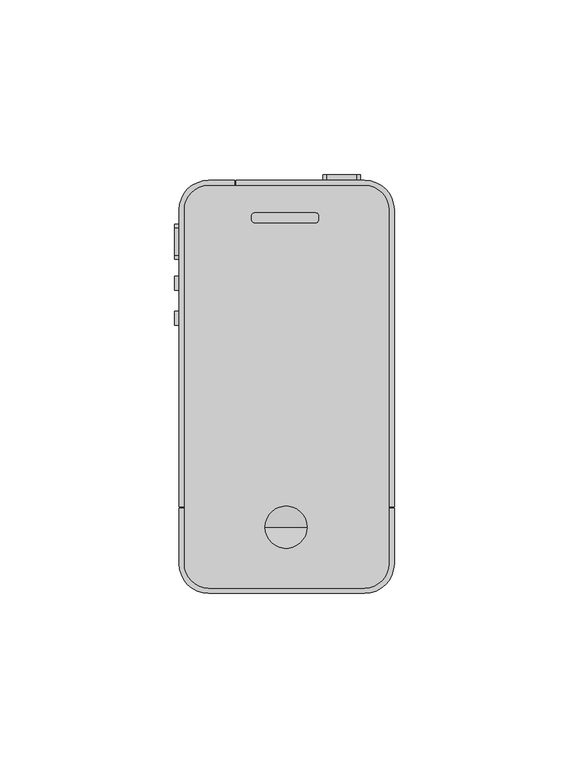
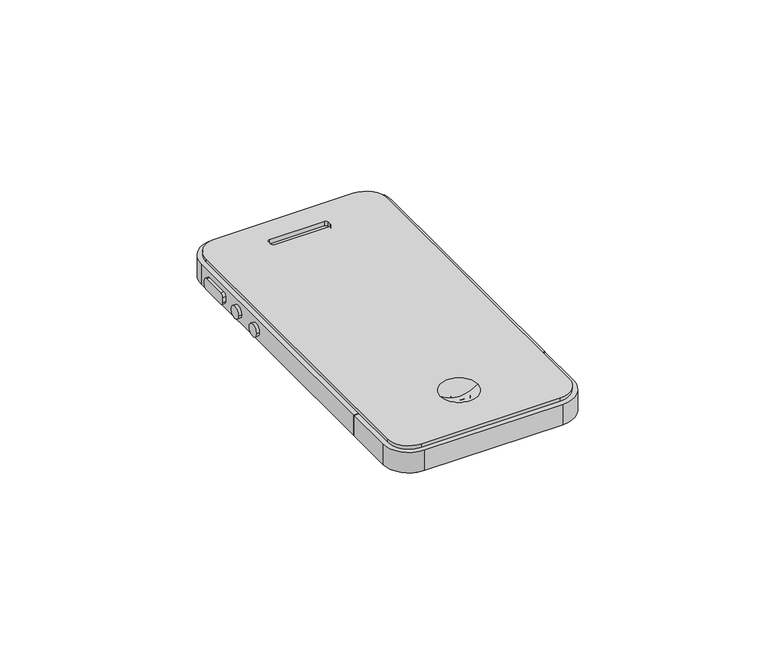
"""IFC4 building model written with IfcOpenShell, lengths in millimetres: furniture geometry."""

from ifc_helpers import new_model, si_unit, point, frame, frame_2d, origin, origin_with_axes, place, context, project, spatial, polyline, circle_curve, ellipse_curve, trimmed, segment, composite_curve, outline, extrude, source, transform, mapped, element, save
from ifc_brep_helpers import plane_surface, cylinder_surface, revolved_surface, advanced_brep


def furniture_542be15f(model_context):
    return source(origin(), model_context, "Body", "SolidModel", [
        extrude(outline(composite_curve([segment(polyline([(32.0792703, 5.7726386), (30.5792703, 5.7726386), (30.5792703, 90.7726386)]), True, "CONTINUOUS"), segment(trimmed(circle_curve(frame_2d((23.5792703, 90.7726386)), 7.0), [point((30.5792703, 90.7726386))], [point((23.5792703, 97.7726386))], True, "CARTESIAN"), True, "CONTINUOUS"), segment(polyline([(23.5792703, 97.7726386), (-13.2335465, 97.7726386), (-13.2335465, 99.2726386), (23.5792703, 99.2726386)]), True, "CONTINUOUS"), segment(trimmed(circle_curve(frame_2d((23.5792703, 90.7726386)), 8.5), [point((23.5792703, 99.2726386))], [point((32.0792703, 90.7726386))], False, "CARTESIAN"), True, "CONTINUOUS"), segment(polyline([(32.0792703, 90.7726386), (32.0792703, 5.7726386)]), True, "CONTINUOUS")], self_intersect=False)), frame((0.0, 0.0, 1.1), z_axis=(0.0, 0.0, 1.0), x_axis=(1.0, 0.0, 0.0)), (0.0, 0.0, 1.0), 7.0),
        extrude(outline(composite_curve([segment(polyline([(-29.5207297, 5.3622902), (-28.0207297, 5.3622902), (-28.0207297, -10.4273614)]), True, "CONTINUOUS"), segment(trimmed(circle_curve(frame_2d((-21.0207297, -10.4273614)), 7.0), [point((-28.0207297, -10.4273614))], [point((-21.0207297, -17.4273614))], True, "CARTESIAN"), True, "CONTINUOUS"), segment(polyline([(-21.0207297, -17.4273614), (23.5792703, -17.4273614)]), True, "CONTINUOUS"), segment(trimmed(circle_curve(frame_2d((23.5792703, -10.4273614)), 7.0), [point((23.5792703, -17.4273614))], [point((30.5792703, -10.4273614))], True, "CARTESIAN"), True, "CONTINUOUS"), segment(polyline([(30.5792703, -10.4273614), (30.5792703, 5.3622902), (32.0792703, 5.3622902), (32.0792703, -10.4273614)]), True, "CONTINUOUS"), segment(trimmed(circle_curve(frame_2d((23.5792703, -10.4273614)), 8.5), [point((32.0792703, -10.4273614))], [point((23.5792703, -18.9273614))], False, "CARTESIAN"), True, "CONTINUOUS"), segment(polyline([(23.5792703, -18.9273614), (-21.0207297, -18.9273614)]), True, "CONTINUOUS"), segment(trimmed(circle_curve(frame_2d((-21.0207297, -10.4273614)), 8.5), [point((-21.0207297, -18.9273614))], [point((-29.5207297, -10.4273614))], False, "CARTESIAN"), True, "CONTINUOUS"), segment(polyline([(-29.5207297, -10.4273614), (-29.5207297, 5.3622902)]), True, "CONTINUOUS")], self_intersect=False)), frame((0.0, 0.0, 1.1), z_axis=(0.0, 0.0, 1.0), x_axis=(1.0, 0.0, 0.0)), (0.0, 0.0, 1.0), 7.0),
        extrude(outline(composite_curve([segment(polyline([(-13.7116671, 99.2726386), (-13.7116671, 97.7726386), (-21.0207297, 97.7726386)]), True, "CONTINUOUS"), segment(trimmed(circle_curve(frame_2d((-21.0207297, 90.7726386)), 7.0), [point((-21.0207297, 97.7726386))], [point((-28.0207297, 90.7726386))], True, "CARTESIAN"), True, "CONTINUOUS"), segment(polyline([(-28.0207297, 90.7726386), (-28.0207297, 5.7726386), (-29.5207297, 5.7726386), (-29.5207297, 90.7726386)]), True, "CONTINUOUS"), segment(trimmed(circle_curve(frame_2d((-21.0207297, 90.7726386)), 8.5), [point((-29.5207297, 90.7726386))], [point((-21.0207297, 99.2726386))], False, "CARTESIAN"), True, "CONTINUOUS"), segment(polyline([(-21.0207297, 99.2726386), (-13.7116671, 99.2726386)]), True, "CONTINUOUS")], self_intersect=False)), frame((0.0, 0.0, 1.1), z_axis=(0.0, 0.0, 1.0), x_axis=(1.0, 0.0, 0.0)), (0.0, 0.0, 1.0), 7.0),
        extrude(outline(composite_curve([segment(trimmed(circle_curve(frame_2d((69.7820043, 4.7126556)), 2.0), [point((71.7820043, 4.7126556))], [point((67.7820043, 4.7126556))], False, "CARTESIAN"), True, "CONTINUOUS"), segment(trimmed(circle_curve(frame_2d((69.7820043, 4.7126556)), 2.0), [point((67.7820043, 4.7126556))], [point((71.7820043, 4.7126556))], False, "CARTESIAN"), True, "CONTINUOUS")], self_intersect=False)), frame((-30.8259803, 0.0, 0.0), z_axis=(1.0, 0.0, 0.0), x_axis=(0.0, 1.0, 0.0)), (0.0, 0.0, 1.0), 1.3052506),
        extrude(outline(composite_curve([segment(trimmed(circle_curve(frame_2d((59.7820043, 4.7126556)), 2.0), [point((61.7820043, 4.7126556))], [point((57.7820043, 4.7126556))], False, "CARTESIAN"), True, "CONTINUOUS"), segment(trimmed(circle_curve(frame_2d((59.7820043, 4.7126556)), 2.0), [point((57.7820043, 4.7126556))], [point((61.7820043, 4.7126556))], False, "CARTESIAN"), True, "CONTINUOUS")], self_intersect=False)), frame((-30.8259803, 0.0, 0.0), z_axis=(1.0, 0.0, 0.0), x_axis=(0.0, 1.0, 0.0)), (0.0, 0.0, 1.0), 1.3052506),
        extrude(outline(composite_curve([segment(polyline([(77.7168489, 6.5044976), (85.7168489, 6.5044976)]), True, "CONTINUOUS"), segment(trimmed(circle_curve(frame_2d((85.7168489, 5.5044976)), 1.0), [point((85.7168489, 6.5044976))], [point((86.7168489, 5.5044976))], False, "CARTESIAN"), True, "CONTINUOUS"), segment(polyline([(86.7168489, 5.5044976), (86.7168489, 3.7684224)]), True, "CONTINUOUS"), segment(trimmed(circle_curve(frame_2d((85.7168489, 3.7684224)), 1.0), [point((86.7168489, 3.7684224))], [point((85.7168489, 2.7684224))], False, "CARTESIAN"), True, "CONTINUOUS"), segment(polyline([(85.7168489, 2.7684224), (77.7168489, 2.7684224)]), True, "CONTINUOUS"), segment(trimmed(circle_curve(frame_2d((77.7168489, 3.7684224)), 1.0), [point((77.7168489, 2.7684224))], [point((76.7168489, 3.7684224))], False, "CARTESIAN"), True, "CONTINUOUS"), segment(polyline([(76.7168489, 3.7684224), (76.7168489, 5.5044976)]), True, "CONTINUOUS"), segment(trimmed(circle_curve(frame_2d((77.7168489, 5.5044976)), 1.0), [point((76.7168489, 5.5044976))], [point((77.7168489, 6.5044976))], False, "CARTESIAN"), True, "CONTINUOUS")], self_intersect=False)), frame((-30.8259803, 0.0, 0.0), z_axis=(1.0, 0.0, 0.0), x_axis=(0.0, 1.0, 0.0)), (0.0, 0.0, 1.0), 1.3052506),
        extrude(outline(composite_curve([segment(trimmed(circle_curve(frame_2d((5.2858186, 12.677609)), 1.0), [point((6.2858186, 12.677609))], [point((5.2858186, 11.677609))], False, "CARTESIAN"), True, "CONTINUOUS"), segment(polyline([(5.2858186, 11.677609), (3.7083939, 11.677609)]), True, "CONTINUOUS"), segment(trimmed(circle_curve(frame_2d((3.7083939, 12.677609)), 1.0), [point((3.7083939, 11.677609))], [point((2.7083939, 12.677609))], False, "CARTESIAN"), True, "CONTINUOUS"), segment(polyline([(2.7083939, 12.677609), (2.7083939, 21.4098831)]), True, "CONTINUOUS"), segment(trimmed(circle_curve(frame_2d((3.7083939, 21.4098831)), 1.0), [point((2.7083939, 21.4098831))], [point((3.7083939, 22.4098831))], False, "CARTESIAN"), True, "CONTINUOUS"), segment(polyline([(3.7083939, 22.4098831), (5.2858186, 22.4098831)]), True, "CONTINUOUS"), segment(trimmed(circle_curve(frame_2d((5.2858186, 21.4098831)), 1.0), [point((5.2858186, 22.4098831))], [point((6.2858186, 21.4098831))], False, "CARTESIAN"), True, "CONTINUOUS"), segment(polyline([(6.2858186, 21.4098831), (6.2858186, 12.677609)]), True, "CONTINUOUS")], self_intersect=False)), frame((0.0, 99.2726386, 0.0), z_axis=(0.0, 1.0, 0.0), x_axis=(0.0, 0.0, 1.0)), (0.0, 0.0, 1.0), 1.595353),
        advanced_brep(
        [(23.5792703, 97.7726386, 9.3), (-21.0207297, 97.7726386, 9.3), (-28.0207297, 90.7726386, 9.3), (-28.0207297, -10.4273614, 9.3), (-21.0207297, -17.4273614, 9.3), (23.5792703, -17.4273614, 9.3), (30.5792703, -10.4273614, 9.3), (30.5792703, 90.7726386, 9.3), (-7.9275969, 89.9216705, 9.3), (9.6036276, 89.9216705, 9.3), (10.4036276, 89.1216705, 9.3), (10.4036276, 87.9700256, 9.3), (9.6036276, 87.1700256, 9.3), (-7.9275969, 87.1700256, 9.3), (-8.7275969, 87.9700256, 9.3), (-8.7275969, 89.1216705, 9.3), (-4.8467871, 0.0, 9.3), (7.1532129, 0.0, 9.3), (23.5792703, 97.7726386, 5.1204413), (30.5792703, 90.7726386, 5.1204413), (30.5792703, -10.4273614, 5.1204413), (23.5792703, -17.4273614, 5.1204413), (-21.0207297, -17.4273614, 5.1204413), (-28.0207297, -10.4273614, 5.1204413), (-28.0207297, 90.7726386, 5.1204413), (-21.0207297, 97.7726386, 5.1204413), (9.6036276, 89.9216705, 7.732621), (-7.9275969, 89.9216705, 7.732621), (-8.7275969, 89.1216705, 7.732621), (-8.7275969, 87.9700256, 7.732621), (-7.9275969, 87.1700256, 7.732621), (9.6036276, 87.1700256, 7.732621), (10.4036276, 87.9700256, 7.732621), (10.4036276, 89.1216705, 7.732621), (1.1532129, 0.0, 7.2033565)],
        [
            (0, 1),
            (1, 2, circle_curve(frame((-21.0207297, 90.7726386, 9.3), z_axis=(0.0, 0.0, 1.0), x_axis=(1.0, 0.0, 0.0)), 7.0)),
            (2, 3),
            (3, 4, circle_curve(frame((-21.0207297, -10.4273614, 9.3), z_axis=(0.0, 0.0, 1.0), x_axis=(1.0, 0.0, 0.0)), 7.0)),
            (4, 5),
            (5, 6, circle_curve(frame((23.5792703, -10.4273614, 9.3), z_axis=(0.0, 0.0, 1.0), x_axis=(1.0, 0.0, 0.0)), 7.0)),
            (6, 7),
            (7, 0, circle_curve(frame((23.5792703, 90.7726386, 9.3), z_axis=(0.0, 0.0, 1.0), x_axis=(1.0, 0.0, 0.0)), 7.0)),
            (8, 9),
            (9, 10, circle_curve(frame((9.6036276, 89.1216705, 9.3), z_axis=(0.0, 0.0, -1.0), x_axis=(1.0, 0.0, 0.0)), 0.8)),
            (10, 11),
            (11, 12, circle_curve(frame((9.6036276, 87.9700256, 9.3), z_axis=(0.0, 0.0, -1.0), x_axis=(1.0, 0.0, 0.0)), 0.8)),
            (12, 13),
            (13, 14, circle_curve(frame((-7.9275969, 87.9700256, 9.3), z_axis=(0.0, 0.0, -1.0), x_axis=(1.0, 0.0, 0.0)), 0.8)),
            (14, 15),
            (15, 8, circle_curve(frame((-7.9275969, 89.1216705, 9.3), z_axis=(0.0, 0.0, -1.0), x_axis=(1.0, 0.0, 0.0)), 0.8)),
            (16, 17, circle_curve(frame((1.1532129, 0.0, 9.3), z_axis=(0.0, 0.0, -1.0), x_axis=(1.0, 0.0, 0.0)), 6.0)),
            (17, 16, circle_curve(frame((1.1532129, 0.0, 9.3), z_axis=(0.0, 0.0, -1.0), x_axis=(1.0, 0.0, 0.0)), 6.0)),
            (18, 19, circle_curve(frame((23.5792703, 90.7726386, 5.1204413), z_axis=(0.0, 0.0, -1.0), x_axis=(1.0, 0.0, 0.0)), 7.0)),
            (19, 20),
            (20, 21, circle_curve(frame((23.5792703, -10.4273614, 5.1204413), z_axis=(0.0, 0.0, -1.0), x_axis=(1.0, 0.0, 0.0)), 7.0)),
            (21, 22),
            (22, 23, circle_curve(frame((-21.0207297, -10.4273614, 5.1204413), z_axis=(0.0, 0.0, -1.0), x_axis=(1.0, 0.0, 0.0)), 7.0)),
            (23, 24),
            (24, 25, circle_curve(frame((-21.0207297, 90.7726386, 5.1204413), z_axis=(0.0, 0.0, -1.0), x_axis=(1.0, 0.0, 0.0)), 7.0)),
            (25, 18),
            (0, 18),
            (25, 1),
            (24, 2),
            (23, 3),
            (22, 4),
            (21, 5),
            (20, 6),
            (19, 7),
            (26, 27),
            (27, 28, circle_curve(frame((-7.9275969, 89.1216705, 7.732621), z_axis=(0.0, 0.0, 1.0), x_axis=(1.0, 0.0, 0.0)), 0.8)),
            (28, 29),
            (29, 30, circle_curve(frame((-7.9275969, 87.9700256, 7.732621), z_axis=(0.0, 0.0, 1.0), x_axis=(1.0, 0.0, 0.0)), 0.8)),
            (30, 31),
            (31, 32, circle_curve(frame((9.6036276, 87.9700256, 7.732621), z_axis=(0.0, 0.0, 1.0), x_axis=(1.0, 0.0, 0.0)), 0.8)),
            (32, 33),
            (33, 26, circle_curve(frame((9.6036276, 89.1216705, 7.732621), z_axis=(0.0, 0.0, 1.0), x_axis=(1.0, 0.0, 0.0)), 0.8)),
            (26, 9),
            (8, 27),
            (15, 28),
            (14, 29),
            (13, 30),
            (12, 31),
            (11, 32),
            (10, 33),
            (16, 34, circle_curve(frame((1.1532129, 0.0, 16.8368289), z_axis=(0.0, -1.0, 0.0), x_axis=(-1.0, 0.0, 0.0)), 9.6334724)),
            (34, 17, circle_curve(frame((1.1532129, 0.0, 16.8368289), z_axis=(0.0, -1.0, 0.0), x_axis=(1.0, 0.0, 0.0)), 9.6334724)),
        ],
        [
            plane_surface(frame((-28.0207297, 97.7726386, 9.3), z_axis=(0.0, 0.0, 1.0), x_axis=(-1.0, 0.0, 0.0))),
            plane_surface(frame((-28.0207297, 97.7726386, 5.1204413), z_axis=(0.0, 0.0, -1.0), x_axis=(1.0, 0.0, 0.0))),
            plane_surface(frame((23.5792703, 97.7726386, 9.3), z_axis=(0.0, 1.0, 0.0), x_axis=(0.0, 0.0, -1.0))),
            cylinder_surface(frame((-21.0207297, 90.7726386, 5.1204413), z_axis=(0.0, 0.0, 1.0), x_axis=(1.0, 0.0, 0.0)), 7.0),
            plane_surface(frame((-28.0207297, 90.7726386, 9.3), z_axis=(-1.0, 0.0, 0.0), x_axis=(0.0, 0.0, -1.0))),
            cylinder_surface(frame((-21.0207297, -10.4273614, 5.1204413), z_axis=(0.0, 0.0, 1.0), x_axis=(1.0, 0.0, 0.0)), 7.0),
            plane_surface(frame((-21.0207297, -17.4273614, 9.3), z_axis=(0.0, -1.0, 0.0), x_axis=(0.0, 0.0, -1.0))),
            cylinder_surface(frame((23.5792703, -10.4273614, 5.1204413), z_axis=(0.0, 0.0, 1.0), x_axis=(1.0, 0.0, 0.0)), 7.0),
            plane_surface(frame((30.5792703, -10.4273614, 9.3), z_axis=(1.0, 0.0, 0.0), x_axis=(0.0, 0.0, -1.0))),
            cylinder_surface(frame((23.5792703, 90.7726386, 5.1204413), z_axis=(0.0, 0.0, 1.0), x_axis=(1.0, 0.0, 0.0)), 7.0),
            plane_surface(frame((-8.7275969, 89.9216705, 7.732621), z_axis=(0.0, 0.0, 1.0), x_axis=(1.0, 0.0, 0.0))),
            plane_surface(frame((9.6036276, 89.9216705, 9.3), z_axis=(0.0, -1.0, 0.0), x_axis=(0.0, 0.0, -1.0))),
            revolved_surface(polyline([(-7.1275969, 89.1216705, 9.3), (-7.1275969, 89.1216705, 7.732621)]), (-7.9275969, 89.1216705, 7.732621), (0.0, 0.0, 1.0)),
            plane_surface(frame((-8.7275969, 89.1216705, 9.3), z_axis=(1.0, 0.0, 0.0), x_axis=(0.0, 0.0, -1.0))),
            revolved_surface(polyline([(-7.1275969, 87.9700256, 9.3), (-7.1275969, 87.9700256, 7.732621)]), (-7.9275969, 87.9700256, 7.732621), (0.0, 0.0, 1.0)),
            plane_surface(frame((-7.9275969, 87.1700256, 9.3), z_axis=(0.0, 1.0, 0.0), x_axis=(0.0, 0.0, -1.0))),
            revolved_surface(polyline([(10.4036276, 87.9700256, 9.3), (10.4036276, 87.9700256, 7.732621)]), (9.6036276, 87.9700256, 7.732621), (0.0, 0.0, 1.0)),
            plane_surface(frame((10.4036276, 87.9700256, 9.3), z_axis=(-1.0, 0.0, 0.0), x_axis=(0.0, 0.0, -1.0))),
            revolved_surface(polyline([(10.4036276, 89.1216705, 9.3), (10.4036276, 89.1216705, 7.732621)]), (9.6036276, 89.1216705, 7.732621), (0.0, 0.0, 1.0)),
            revolved_surface(trimmed(ellipse_curve(frame((1.1532129, 0.0, 16.8368289), z_axis=(0.0, 1.0, 0.0), x_axis=(1.0, 0.0, 0.0)), 9.6334724, 9.6334724), [point((7.1532129, 0.0, 9.3))], [point((1.1532129, 0.0, 7.2033565))], True, "CARTESIAN"), (1.1532129, 0.0, 9.3), (0.0, 0.0, 1.0)),
        ],
        [
            (0, [[1, 2, 3, 4, 5, 6, 7, 8], [9, 10, 11, 12, 13, 14, 15, 16], [17, 18]]),
            (1, [[19, 20, 21, 22, 23, 24, 25, 26]]),
            (2, [[-1, 27, -26, 28]]),
            (3, [[-2, -28, -25, 29]]),
            (4, [[-3, -29, -24, 30]]),
            (5, [[-4, -30, -23, 31]]),
            (6, [[-5, -31, -22, 32]]),
            (7, [[-6, -32, -21, 33]]),
            (8, [[-7, -33, -20, 34]]),
            (9, [[-8, -34, -19, -27]]),
            (10, [[35, 36, 37, 38, 39, 40, 41, 42]]),
            (11, [[-35, 43, -9, 44]]),
            (12, [[-36, -44, -16, 45]]),
            (13, [[-37, -45, -15, 46]]),
            (14, [[-38, -46, -14, 47]]),
            (15, [[-39, -47, -13, 48]]),
            (16, [[-40, -48, -12, 49]]),
            (17, [[-41, -49, -11, 50]]),
            (18, [[-42, -50, -10, -43]]),
            (19, [[51, 52, -17]]),
            (19, [[-51, -18, -52]]),
        ],
    ),
        extrude(outline(composite_curve([segment(polyline([(-7.9275969, 89.9216705), (9.6036276, 89.9216705)]), True, "CONTINUOUS"), segment(trimmed(circle_curve(frame_2d((9.6036276, 89.1216705)), 0.8), [point((9.6036276, 89.9216705))], [point((10.4036276, 89.1216705))], False, "CARTESIAN"), True, "CONTINUOUS"), segment(polyline([(10.4036276, 89.1216705), (10.4036276, 87.9700256)]), True, "CONTINUOUS"), segment(trimmed(circle_curve(frame_2d((9.6036276, 87.9700256)), 0.8), [point((10.4036276, 87.9700256))], [point((9.6036276, 87.1700256))], False, "CARTESIAN"), True, "CONTINUOUS"), segment(polyline([(9.6036276, 87.1700256), (-7.9275969, 87.1700256)]), True, "CONTINUOUS"), segment(trimmed(circle_curve(frame_2d((-7.9275969, 87.9700256)), 0.8), [point((-7.9275969, 87.1700256))], [point((-8.7275969, 87.9700256))], False, "CARTESIAN"), True, "CONTINUOUS"), segment(polyline([(-8.7275969, 87.9700256), (-8.7275969, 89.1216705)]), True, "CONTINUOUS"), segment(trimmed(circle_curve(frame_2d((-7.9275969, 89.1216705)), 0.8), [point((-8.7275969, 89.1216705))], [point((-7.9275969, 89.9216705))], False, "CARTESIAN"), True, "CONTINUOUS")], self_intersect=False)), frame((0.0, 0.0, 5.1204413), z_axis=(0.0, 0.0, 1.0), x_axis=(1.0, 0.0, 0.0)), (0.0, 0.0, 1.0), 2.9795587),
        extrude(outline(composite_curve([segment(trimmed(circle_curve(frame_2d((23.5792703, 90.7726386)), 7.0), [point((23.5792703, 97.7726386))], [point((30.5792703, 90.7726386))], False, "CARTESIAN"), True, "CONTINUOUS"), segment(polyline([(30.5792703, 90.7726386), (30.5792703, -10.4273614)]), True, "CONTINUOUS"), segment(trimmed(circle_curve(frame_2d((23.5792703, -10.4273614)), 7.0), [point((30.5792703, -10.4273614))], [point((23.5792703, -17.4273614))], False, "CARTESIAN"), True, "CONTINUOUS"), segment(polyline([(23.5792703, -17.4273614), (-21.0207297, -17.4273614)]), True, "CONTINUOUS"), segment(trimmed(circle_curve(frame_2d((-21.0207297, -10.4273614)), 7.0), [point((-21.0207297, -17.4273614))], [point((-28.0207297, -10.4273614))], False, "CARTESIAN"), True, "CONTINUOUS"), segment(polyline([(-28.0207297, -10.4273614), (-28.0207297, 90.7726386)]), True, "CONTINUOUS"), segment(trimmed(circle_curve(frame_2d((-21.0207297, 90.7726386)), 7.0), [point((-28.0207297, 90.7726386))], [point((-21.0207297, 97.7726386))], False, "CARTESIAN"), True, "CONTINUOUS"), segment(polyline([(-21.0207297, 97.7726386), (23.5792703, 97.7726386)]), True, "CONTINUOUS")], self_intersect=False)), origin_with_axes(), (0.0, 0.0, 1.0), 5.1204413),
        extrude(outline(composite_curve([segment(trimmed(circle_curve(frame_2d((2.7857533, 1.5951851)), 1.6), [point((2.7857533, 3.1951851))], [point((4.3857533, 1.5951851))], False, "CARTESIAN"), True, "CONTINUOUS"), segment(polyline([(4.3857533, 1.5951851), (4.3857533, -1.7262558)]), True, "CONTINUOUS"), segment(trimmed(circle_curve(frame_2d((2.7857533, -1.7262558)), 1.6), [point((4.3857533, -1.7262558))], [point((2.7857533, -3.3262558))], False, "CARTESIAN"), True, "CONTINUOUS"), segment(polyline([(2.7857533, -3.3262558), (-0.5142467, -3.3262558)]), True, "CONTINUOUS"), segment(trimmed(circle_curve(frame_2d((-0.5142467, -1.7262558)), 1.6), [point((-0.5142467, -3.3262558))], [point((-2.1142467, -1.7262558))], False, "CARTESIAN"), True, "CONTINUOUS"), segment(polyline([(-2.1142467, -1.7262558), (-2.1142467, 1.5951851)]), True, "CONTINUOUS"), segment(trimmed(circle_curve(frame_2d((-0.5142467, 1.5951851)), 1.6), [point((-2.1142467, 1.5951851))], [point((-0.5142467, 3.1951851))], False, "CARTESIAN"), True, "CONTINUOUS"), segment(polyline([(-0.5142467, 3.1951851), (2.7857533, 3.1951851)]), True, "CONTINUOUS")], self_intersect=False), holes=[composite_curve([segment(polyline([(2.7857533, 2.3951851), (-0.5142467, 2.3951851)]), True, "CONTINUOUS"), segment(trimmed(circle_curve(frame_2d((-0.5142467, 1.5951851)), 0.8), [point((-0.5142467, 2.3951851))], [point((-1.3142467, 1.5951851))], True, "CARTESIAN"), True, "CONTINUOUS"), segment(polyline([(-1.3142467, 1.5951851), (-1.3142467, -1.7262558)]), True, "CONTINUOUS"), segment(trimmed(circle_curve(frame_2d((-0.5142467, -1.7262558)), 0.8), [point((-1.3142467, -1.7262558))], [point((-0.5142467, -2.5262558))], True, "CARTESIAN"), True, "CONTINUOUS"), segment(polyline([(-0.5142467, -2.5262558), (2.7857533, -2.5262558)]), True, "CONTINUOUS"), segment(trimmed(circle_curve(frame_2d((2.7857533, -1.7262558)), 0.8), [point((2.7857533, -2.5262558))], [point((3.5857533, -1.7262558))], True, "CARTESIAN"), True, "CONTINUOUS"), segment(polyline([(3.5857533, -1.7262558), (3.5857533, 1.5951851)]), True, "CONTINUOUS"), segment(trimmed(circle_curve(frame_2d((2.7857533, 1.5951851)), 0.8), [point((3.5857533, 1.5951851))], [point((2.7857533, 2.3951851))], True, "CARTESIAN"), True, "CONTINUOUS")], self_intersect=False)]), frame((0.0, 0.0, 6.1536863), z_axis=(0.0, 0.0, 1.0), x_axis=(1.0, 0.0, 0.0)), (0.0, 0.0, 1.0), 1.6778761),
    ])


if __name__ == "__main__":
    model = new_model("IFC4")
    model_context = context("Model", 3, world=origin())
    ifc_project = project(units=[si_unit("LENGTHUNIT", "METRE", prefix="MILLI")], contexts=[model_context])
    site = spatial("IfcSite", under=ifc_project)
    building = spatial("IfcBuilding", under=site)
    placement = place(None, origin())
    furniture_shape = furniture_542be15f(model_context)
    element("IfcFurniture", 1, at=placement, inside=building, context=model_context, shape_type="MappedRepresentation", body=[
        mapped(furniture_shape, transform((0.0, 0.0, 0.0), x_axis=(1.0, 0.0, 0.0), y_axis=(0.0, 1.0, 0.0), z_axis=(0.0, 0.0, 1.0))),
    ])
    save(model, "model.ifc")

# Revit data of these elements
# Type
#   Default Elevation = 0
